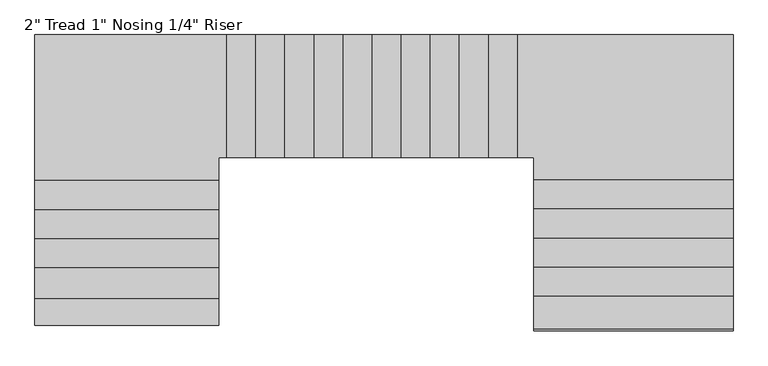
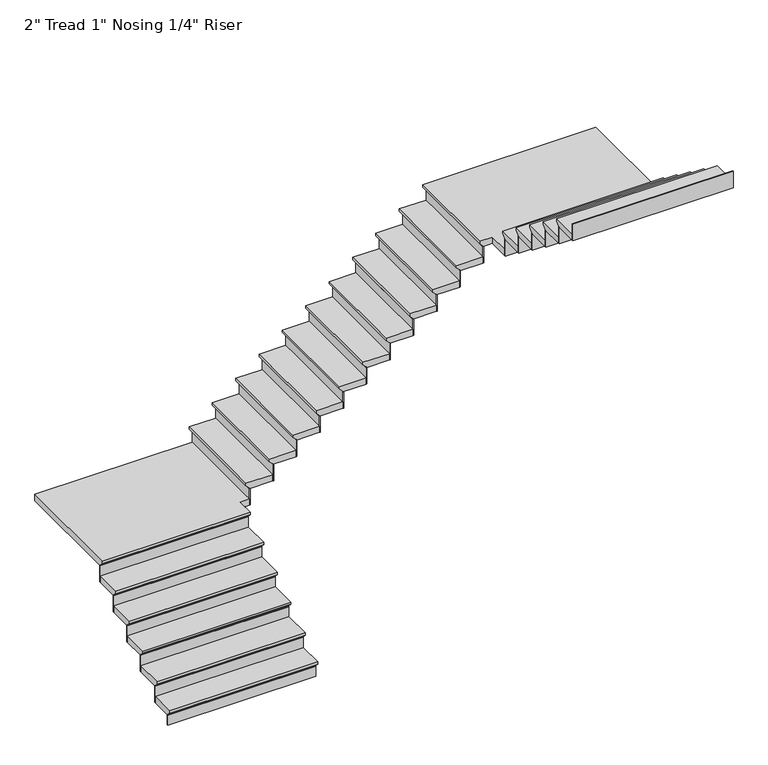
"""IFC4 building model written with IfcOpenShell, lengths in millimetres: stair flight geometry."""

from ifc_helpers import new_model, si_unit, origin, place, context, project, spatial, faceted_brep, source, transform, mapped, element, save


def stair_flight_d1d5caa0(model_context):
    return source(origin(), model_context, "Body", "Brep", [
        faceted_brep([(-2368.6972892, 4718.9167606, 3313.8717391), (-2368.6972892, 4718.9167606, 3332.9217391), (-3493.0046642, 4718.9167606, 3332.9217391), (-3493.0046642, 4718.9167606, 3313.8717391), (-2368.6972892, 4744.3167606, 3288.4717391), (-3493.0046642, 4744.3167606, 3288.4717391), (-2368.6972892, 4909.4167606, 3332.9217391), (-3493.0046642, 4909.4167606, 3332.9217391), (-3493.0046642, 4744.3167606, 3282.1217391), (-3493.0046642, 4909.4167606, 3282.1217391), (-2368.6972892, 4909.4167606, 3282.1217391), (-2368.6972892, 4744.3167606, 3282.1217391)], [[[0, 1, 2, 3]], [[4, 0, 3, 5]], [[2, 1, 6, 7]], [[8, 9, 10, 11]], [[2, 7, 9, 8, 5, 3]], [[8, 11, 4, 5]], [[6, 1, 0, 4, 11, 10]], [[7, 6, 10, 9]]]),
        faceted_brep([(-2368.6972892, 4744.3167606, 3282.1217391), (-2368.6972892, 4744.3167606, 3200.4), (-2368.6972892, 4750.6667606, 3200.4), (-2368.6972892, 4750.6667606, 3282.1217391), (-3493.0046642, 4744.3167606, 3282.1217391), (-3493.0046642, 4750.6667606, 3282.1217391), (-3493.0046642, 4750.6667606, 3200.4), (-3493.0046642, 4744.3167606, 3200.4)], [[[0, 1, 2, 3]], [[4, 5, 6, 7]], [[1, 0, 4, 7]], [[2, 1, 7, 6]], [[3, 2, 6, 5]], [[0, 3, 5, 4]]]),
        faceted_brep([(-2368.6972892, 4909.4167606, 3414.6434783), (-2368.6972892, 4909.4167606, 3282.1217391), (-2368.6972892, 4915.7667606, 3282.1217391), (-2368.6972892, 4915.7667606, 3414.6434783), (-3493.0046642, 4909.4167606, 3414.6434783), (-3493.0046642, 4915.7667606, 3414.6434783), (-3493.0046642, 4915.7667606, 3282.1217391), (-3493.0046642, 4909.4167606, 3282.1217391)], [[[0, 1, 2, 3]], [[4, 5, 6, 7]], [[1, 0, 4, 7]], [[2, 1, 7, 6]], [[3, 2, 6, 5]], [[0, 3, 5, 4]]]),
        faceted_brep([(-3493.0046642, 4884.0167606, 3465.4434783), (-2368.6972892, 4884.0167606, 3465.4434783), (-2368.6972892, 5099.9164494, 3465.4434783), (-3493.0046642, 5099.9164494, 3465.4434783), (-3493.0046642, 4909.4167606, 3414.6434783), (-3493.0046642, 5099.9164494, 3414.6434783), (-2368.6972892, 5099.9164494, 3414.6434783), (-2368.6972892, 4909.4167606, 3414.6434783), (-3493.0046642, 4909.4167606, 3420.9934783), (-3493.0046642, 4884.0167606, 3446.3934783), (-2368.6972892, 4909.4167606, 3420.9934783), (-2368.6972892, 4884.0167606, 3446.3934783)], [[[0, 1, 2, 3]], [[4, 5, 6, 7]], [[0, 3, 5, 4, 8, 9]], [[4, 7, 10, 8]], [[2, 1, 11, 10, 7, 6]], [[3, 2, 6, 5]], [[11, 1, 0, 9]], [[10, 11, 9, 8]]]),
        faceted_brep([(-2368.6972892, 5099.9164494, 3547.1652174), (-2368.6972892, 5099.9164494, 3414.6434783), (-2368.6972892, 5106.2664494, 3414.6434783), (-2368.6972892, 5106.2664494, 3547.1652174), (-3493.0046642, 5099.9164494, 3547.1652174), (-3493.0046642, 5106.2664494, 3547.1652174), (-3493.0046642, 5106.2664494, 3414.6434783), (-3493.0046642, 5099.9164494, 3414.6434783)], [[[0, 1, 2, 3]], [[4, 5, 6, 7]], [[1, 0, 4, 7]], [[2, 1, 7, 6]], [[3, 2, 6, 5]], [[0, 3, 5, 4]]]),
        faceted_brep([(-3493.0046642, 5074.5164494, 3597.9652174), (-2368.6972892, 5074.5164494, 3597.9652174), (-2368.6972892, 5277.7164494, 3597.9652174), (-3493.0046642, 5277.7164494, 3597.9652174), (-3493.0046642, 5099.9164494, 3547.1652174), (-3493.0046642, 5277.7164494, 3547.1652174), (-2368.6972892, 5277.7164494, 3547.1652174), (-2368.6972892, 5099.9164494, 3547.1652174), (-3493.0046642, 5099.9164494, 3553.5152174), (-3493.0046642, 5074.5164494, 3578.9152174), (-2368.6972892, 5099.9164494, 3553.5152174), (-2368.6972892, 5074.5164494, 3578.9152174)], [[[0, 1, 2, 3]], [[4, 5, 6, 7]], [[0, 3, 5, 4, 8, 9]], [[4, 7, 10, 8]], [[2, 1, 11, 10, 7, 6]], [[3, 2, 6, 5]], [[11, 1, 0, 9]], [[10, 11, 9, 8]]]),
        faceted_brep([(-2368.6972892, 5277.7164494, 3679.6869565), (-2368.6972892, 5277.7164494, 3547.1652174), (-2368.6972892, 5284.0664494, 3547.1652174), (-2368.6972892, 5284.0664494, 3679.6869565), (-3493.0046642, 5277.7164494, 3679.6869565), (-3493.0046642, 5284.0664494, 3679.6869565), (-3493.0046642, 5284.0664494, 3547.1652174), (-3493.0046642, 5277.7164494, 3547.1652174)], [[[0, 1, 2, 3]], [[4, 5, 6, 7]], [[1, 0, 4, 7]], [[2, 1, 7, 6]], [[3, 2, 6, 5]], [[0, 3, 5, 4]]]),
        faceted_brep([(-3493.0046642, 5252.3164494, 3730.4869565), (-2368.6972892, 5252.3164494, 3730.4869565), (-2368.6972892, 5455.5164494, 3730.4869565), (-3493.0046642, 5455.5164494, 3730.4869565), (-3493.0046642, 5277.7164494, 3679.6869565), (-3493.0046642, 5455.5164494, 3679.6869565), (-2368.6972892, 5455.5164494, 3679.6869565), (-2368.6972892, 5277.7164494, 3679.6869565), (-3493.0046642, 5277.7164494, 3686.0369565), (-3493.0046642, 5252.3164494, 3711.4369565), (-2368.6972892, 5277.7164494, 3686.0369565), (-2368.6972892, 5252.3164494, 3711.4369565)], [[[0, 1, 2, 3]], [[4, 5, 6, 7]], [[0, 3, 5, 4, 8, 9]], [[4, 7, 10, 8]], [[2, 1, 11, 10, 7, 6]], [[3, 2, 6, 5]], [[11, 1, 0, 9]], [[10, 11, 9, 8]]]),
        faceted_brep([(-2368.6972892, 5455.5164494, 3812.2086957), (-2368.6972892, 5455.5164494, 3679.6869565), (-2368.6972892, 5461.8664494, 3679.6869565), (-2368.6972892, 5461.8664494, 3812.2086957), (-3493.0046642, 5455.5164494, 3812.2086957), (-3493.0046642, 5461.8664494, 3812.2086957), (-3493.0046642, 5461.8664494, 3679.6869565), (-3493.0046642, 5455.5164494, 3679.6869565)], [[[0, 1, 2, 3]], [[4, 5, 6, 7]], [[1, 0, 4, 7]], [[2, 1, 7, 6]], [[3, 2, 6, 5]], [[0, 3, 5, 4]]]),
        faceted_brep([(-3493.0046642, 5430.1164494, 3863.0086957), (-2368.6972892, 5430.1164494, 3863.0086957), (-2368.6972892, 5633.3167606, 3863.0086957), (-3493.0046642, 5633.3167606, 3863.0086957), (-3493.0046642, 5455.5164494, 3812.2086957), (-3493.0046642, 5633.3167606, 3812.2086957), (-2368.6972892, 5633.3167606, 3812.2086957), (-2368.6972892, 5455.5164494, 3812.2086957), (-3493.0046642, 5455.5164494, 3818.5586957), (-3493.0046642, 5430.1164494, 3843.9586957), (-2368.6972892, 5455.5164494, 3818.5586957), (-2368.6972892, 5430.1164494, 3843.9586957)], [[[0, 1, 2, 3]], [[4, 5, 6, 7]], [[0, 3, 5, 4, 8, 9]], [[4, 7, 10, 8]], [[2, 1, 11, 10, 7, 6]], [[3, 2, 6, 5]], [[11, 1, 0, 9]], [[10, 11, 9, 8]]]),
        faceted_brep([(-2368.6972892, 5633.3167606, 3944.7304348), (-2368.6972892, 5633.3167606, 3812.2086957), (-2368.6972892, 5639.6667606, 3812.2086957), (-2368.6972892, 5639.6667606, 3944.7304348), (-3493.0046642, 5633.3167606, 3944.7304348), (-3493.0046642, 5639.6667606, 3944.7304348), (-3493.0046642, 5639.6667606, 3812.2086957), (-3493.0046642, 5633.3167606, 3812.2086957)], [[[0, 1, 2, 3]], [[4, 5, 6, 7]], [[1, 0, 4, 7]], [[2, 1, 7, 6]], [[3, 2, 6, 5]], [[0, 3, 5, 4]]]),
        faceted_brep([(-2295.032382, 6496.9167606, 3995.5304348), (-3493.0046642, 6496.9167606, 3995.5304348), (-3493.0046642, 5607.9167606, 3995.5304348), (-2368.6972892, 5607.9167606, 3995.5304348), (-2368.6972892, 5746.5536537, 3995.5304348), (-2295.032382, 5746.5536537, 3995.5304348), (-3493.0046642, 6496.9167606, 3944.7304348), (-2295.032382, 6496.9167606, 3944.7304348), (-2295.032382, 5746.5536537, 3944.7304348), (-2368.6972892, 5746.5536537, 3944.7304348), (-2368.6972892, 5633.3167606, 3944.7304348), (-3493.0046642, 5633.3167606, 3944.7304348), (-3493.0046642, 5633.3167606, 3951.0804348), (-3493.0046642, 5607.9167606, 3976.4804348), (-2368.6972892, 5633.3167606, 3951.0804348), (-2368.6972892, 5607.9167606, 3976.4804348)], [[[0, 1, 2, 3, 4, 5]], [[6, 7, 8, 9, 10, 11]], [[1, 0, 7, 6]], [[2, 1, 6, 11, 12, 13]], [[11, 10, 14, 12]], [[4, 3, 15, 14, 10, 9]], [[5, 4, 9, 8]], [[0, 5, 8, 7]], [[15, 3, 2, 13]], [[14, 15, 13, 12]]]),
        faceted_brep([(-2295.032382, 5746.5536537, 4077.2521739), (-2295.032382, 5746.5536537, 3944.7304348), (-2288.682382, 5746.5536537, 3944.7304348), (-2288.682382, 5746.5536537, 4077.2521739), (-2295.032382, 6496.9167606, 4077.2521739), (-2288.682382, 6496.9167606, 4077.2521739), (-2288.682382, 6496.9167606, 3944.7304348), (-2295.032382, 6496.9167606, 3944.7304348)], [[[0, 1, 2, 3]], [[4, 5, 6, 7]], [[1, 0, 4, 7]], [[2, 1, 7, 6]], [[3, 2, 6, 5]], [[0, 3, 5, 4]]]),
        faceted_brep([(-2320.432382, 6496.9167606, 4128.0521739), (-2320.432382, 5746.5536537, 4128.0521739), (-2117.232382, 5746.5536537, 4128.0521739), (-2117.232382, 6496.9167606, 4128.0521739), (-2295.032382, 6496.9167606, 4077.2521739), (-2117.232382, 6496.9167606, 4077.2521739), (-2117.232382, 5746.5536537, 4077.2521739), (-2295.032382, 5746.5536537, 4077.2521739), (-2295.032382, 6496.9167606, 4083.6021739), (-2320.432382, 6496.9167606, 4109.0021739), (-2295.032382, 5746.5536537, 4083.6021739), (-2320.432382, 5746.5536537, 4109.0021739)], [[[0, 1, 2, 3]], [[4, 5, 6, 7]], [[0, 3, 5, 4, 8, 9]], [[4, 7, 10, 8]], [[2, 1, 11, 10, 7, 6]], [[3, 2, 6, 5]], [[11, 1, 0, 9]], [[10, 11, 9, 8]]]),
        faceted_brep([(-2117.232382, 5746.5536537, 4209.773913), (-2117.232382, 5746.5536537, 4077.2521739), (-2110.882382, 5746.5536537, 4077.2521739), (-2110.882382, 5746.5536537, 4209.773913), (-2117.232382, 6496.9167606, 4209.773913), (-2110.882382, 6496.9167606, 4209.773913), (-2110.882382, 6496.9167606, 4077.2521739), (-2117.232382, 6496.9167606, 4077.2521739)], [[[0, 1, 2, 3]], [[4, 5, 6, 7]], [[1, 0, 4, 7]], [[2, 1, 7, 6]], [[3, 2, 6, 5]], [[0, 3, 5, 4]]]),
        faceted_brep([(-2142.632382, 6496.9167606, 4260.573913), (-2142.632382, 5746.5536537, 4260.573913), (-1939.432382, 5746.5536537, 4260.573913), (-1939.432382, 6496.9167606, 4260.573913), (-2117.232382, 6496.9167606, 4209.773913), (-1939.432382, 6496.9167606, 4209.773913), (-1939.432382, 5746.5536537, 4209.773913), (-2117.232382, 5746.5536537, 4209.773913), (-2117.232382, 6496.9167606, 4216.123913), (-2142.632382, 6496.9167606, 4241.523913), (-2117.232382, 5746.5536537, 4216.123913), (-2142.632382, 5746.5536537, 4241.523913)], [[[0, 1, 2, 3]], [[4, 5, 6, 7]], [[0, 3, 5, 4, 8, 9]], [[4, 7, 10, 8]], [[2, 1, 11, 10, 7, 6]], [[3, 2, 6, 5]], [[11, 1, 0, 9]], [[10, 11, 9, 8]]]),
        faceted_brep([(-1939.432382, 5746.5536537, 4342.2956522), (-1939.432382, 5746.5536537, 4209.773913), (-1933.082382, 5746.5536537, 4209.773913), (-1933.082382, 5746.5536537, 4342.2956522), (-1939.432382, 6496.9167606, 4342.2956522), (-1933.082382, 6496.9167606, 4342.2956522), (-1933.082382, 6496.9167606, 4209.773913), (-1939.432382, 6496.9167606, 4209.773913)], [[[0, 1, 2, 3]], [[4, 5, 6, 7]], [[1, 0, 4, 7]], [[2, 1, 7, 6]], [[3, 2, 6, 5]], [[0, 3, 5, 4]]]),
        faceted_brep([(-1964.832382, 6496.9167606, 4393.0956522), (-1964.832382, 5746.5536537, 4393.0956522), (-1761.632382, 5746.5536537, 4393.0956522), (-1761.632382, 6496.9167606, 4393.0956522), (-1939.432382, 6496.9167606, 4342.2956522), (-1761.632382, 6496.9167606, 4342.2956522), (-1761.632382, 5746.5536537, 4342.2956522), (-1939.432382, 5746.5536537, 4342.2956522), (-1939.432382, 6496.9167606, 4348.6456522), (-1964.832382, 6496.9167606, 4374.0456522), (-1939.432382, 5746.5536537, 4348.6456522), (-1964.832382, 5746.5536537, 4374.0456522)], [[[0, 1, 2, 3]], [[4, 5, 6, 7]], [[0, 3, 5, 4, 8, 9]], [[4, 7, 10, 8]], [[2, 1, 11, 10, 7, 6]], [[3, 2, 6, 5]], [[11, 1, 0, 9]], [[10, 11, 9, 8]]]),
        faceted_brep([(-1761.632382, 5746.5536537, 4474.8173913), (-1761.632382, 5746.5536537, 4342.2956522), (-1755.282382, 5746.5536537, 4342.2956522), (-1755.282382, 5746.5536537, 4474.8173913), (-1761.632382, 6496.9167606, 4474.8173913), (-1755.282382, 6496.9167606, 4474.8173913), (-1755.282382, 6496.9167606, 4342.2956522), (-1761.632382, 6496.9167606, 4342.2956522)], [[[0, 1, 2, 3]], [[4, 5, 6, 7]], [[1, 0, 4, 7]], [[2, 1, 7, 6]], [[3, 2, 6, 5]], [[0, 3, 5, 4]]]),
        faceted_brep([(-1787.032382, 6496.9167606, 4525.6173913), (-1787.032382, 5746.5536537, 4525.6173913), (-1583.832382, 5746.5536537, 4525.6173913), (-1583.832382, 6496.9167606, 4525.6173913), (-1761.632382, 6496.9167606, 4474.8173913), (-1583.832382, 6496.9167606, 4474.8173913), (-1583.832382, 5746.5536537, 4474.8173913), (-1761.632382, 5746.5536537, 4474.8173913), (-1761.632382, 6496.9167606, 4481.1673913), (-1787.032382, 6496.9167606, 4506.5673913), (-1761.632382, 5746.5536537, 4481.1673913), (-1787.032382, 5746.5536537, 4506.5673913)], [[[0, 1, 2, 3]], [[4, 5, 6, 7]], [[0, 3, 5, 4, 8, 9]], [[4, 7, 10, 8]], [[2, 1, 11, 10, 7, 6]], [[3, 2, 6, 5]], [[11, 1, 0, 9]], [[10, 11, 9, 8]]]),
        faceted_brep([(-1583.832382, 5746.5536537, 4607.3391304), (-1583.832382, 5746.5536537, 4474.8173913), (-1577.482382, 5746.5536537, 4474.8173913), (-1577.482382, 5746.5536537, 4607.3391304), (-1583.832382, 6496.9167606, 4607.3391304), (-1577.482382, 6496.9167606, 4607.3391304), (-1577.482382, 6496.9167606, 4474.8173913), (-1583.832382, 6496.9167606, 4474.8173913)], [[[0, 1, 2, 3]], [[4, 5, 6, 7]], [[1, 0, 4, 7]], [[2, 1, 7, 6]], [[3, 2, 6, 5]], [[0, 3, 5, 4]]]),
        faceted_brep([(-1609.232382, 6496.9167606, 4658.1391304), (-1609.232382, 5746.5536537, 4658.1391304), (-1406.032382, 5746.5536537, 4658.1391304), (-1406.032382, 6496.9167606, 4658.1391304), (-1583.832382, 6496.9167606, 4607.3391304), (-1406.032382, 6496.9167606, 4607.3391304), (-1406.032382, 5746.5536537, 4607.3391304), (-1583.832382, 5746.5536537, 4607.3391304), (-1583.832382, 6496.9167606, 4613.6891304), (-1609.232382, 6496.9167606, 4639.0891304), (-1583.832382, 5746.5536537, 4613.6891304), (-1609.232382, 5746.5536537, 4639.0891304)], [[[0, 1, 2, 3]], [[4, 5, 6, 7]], [[0, 3, 5, 4, 8, 9]], [[4, 7, 10, 8]], [[2, 1, 11, 10, 7, 6]], [[3, 2, 6, 5]], [[11, 1, 0, 9]], [[10, 11, 9, 8]]]),
        faceted_brep([(-1406.032382, 5746.5536537, 4739.8608696), (-1406.032382, 5746.5536537, 4607.3391304), (-1399.682382, 5746.5536537, 4607.3391304), (-1399.682382, 5746.5536537, 4739.8608696), (-1406.032382, 6496.9167606, 4739.8608696), (-1399.682382, 6496.9167606, 4739.8608696), (-1399.682382, 6496.9167606, 4607.3391304), (-1406.032382, 6496.9167606, 4607.3391304)], [[[0, 1, 2, 3]], [[4, 5, 6, 7]], [[1, 0, 4, 7]], [[2, 1, 7, 6]], [[3, 2, 6, 5]], [[0, 3, 5, 4]]]),
        faceted_brep([(-1431.432382, 6496.9167606, 4790.6608696), (-1431.432382, 5746.5536537, 4790.6608696), (-1228.232382, 5746.5536537, 4790.6608696), (-1228.232382, 6496.9167606, 4790.6608696), (-1406.032382, 6496.9167606, 4739.8608696), (-1228.232382, 6496.9167606, 4739.8608696), (-1228.232382, 5746.5536537, 4739.8608696), (-1406.032382, 5746.5536537, 4739.8608696), (-1406.032382, 6496.9167606, 4746.2108696), (-1431.432382, 6496.9167606, 4771.6108696), (-1406.032382, 5746.5536537, 4746.2108696), (-1431.432382, 5746.5536537, 4771.6108696)], [[[0, 1, 2, 3]], [[4, 5, 6, 7]], [[0, 3, 5, 4, 8, 9]], [[4, 7, 10, 8]], [[2, 1, 11, 10, 7, 6]], [[3, 2, 6, 5]], [[11, 1, 0, 9]], [[10, 11, 9, 8]]]),
        faceted_brep([(-1228.232382, 5746.5536537, 4872.3826087), (-1228.232382, 5746.5536537, 4739.8608696), (-1221.882382, 5746.5536537, 4739.8608696), (-1221.882382, 5746.5536537, 4872.3826087), (-1228.232382, 6496.9167606, 4872.3826087), (-1221.882382, 6496.9167606, 4872.3826087), (-1221.882382, 6496.9167606, 4739.8608696), (-1228.232382, 6496.9167606, 4739.8608696)], [[[0, 1, 2, 3]], [[4, 5, 6, 7]], [[1, 0, 4, 7]], [[2, 1, 7, 6]], [[3, 2, 6, 5]], [[0, 3, 5, 4]]]),
        faceted_brep([(-1253.632382, 6496.9167606, 4923.1826087), (-1253.632382, 5746.5536537, 4923.1826087), (-1050.432382, 5746.5536537, 4923.1826087), (-1050.432382, 6496.9167606, 4923.1826087), (-1228.232382, 6496.9167606, 4872.3826087), (-1050.432382, 6496.9167606, 4872.3826087), (-1050.432382, 5746.5536537, 4872.3826087), (-1228.232382, 5746.5536537, 4872.3826087), (-1228.232382, 6496.9167606, 4878.7326087), (-1253.632382, 6496.9167606, 4904.1326087), (-1228.232382, 5746.5536537, 4878.7326087), (-1253.632382, 5746.5536537, 4904.1326087)], [[[0, 1, 2, 3]], [[4, 5, 6, 7]], [[0, 3, 5, 4, 8, 9]], [[4, 7, 10, 8]], [[2, 1, 11, 10, 7, 6]], [[3, 2, 6, 5]], [[11, 1, 0, 9]], [[10, 11, 9, 8]]]),
        faceted_brep([(-1050.432382, 5746.5536537, 5004.9043478), (-1050.432382, 5746.5536537, 4872.3826087), (-1044.082382, 5746.5536537, 4872.3826087), (-1044.082382, 5746.5536537, 5004.9043478), (-1050.432382, 6496.9167606, 5004.9043478), (-1044.082382, 6496.9167606, 5004.9043478), (-1044.082382, 6496.9167606, 4872.3826087), (-1050.432382, 6496.9167606, 4872.3826087)], [[[0, 1, 2, 3]], [[4, 5, 6, 7]], [[1, 0, 4, 7]], [[2, 1, 7, 6]], [[3, 2, 6, 5]], [[0, 3, 5, 4]]]),
        faceted_brep([(-1075.832382, 6496.9167606, 5055.7043478), (-1075.832382, 5746.5536537, 5055.7043478), (-872.632382, 5746.5536537, 5055.7043478), (-872.632382, 6496.9167606, 5055.7043478), (-1050.432382, 6496.9167606, 5004.9043478), (-872.632382, 6496.9167606, 5004.9043478), (-872.632382, 5746.5536537, 5004.9043478), (-1050.432382, 5746.5536537, 5004.9043478), (-1050.432382, 6496.9167606, 5011.2543478), (-1075.832382, 6496.9167606, 5036.6543478), (-1050.432382, 5746.5536537, 5011.2543478), (-1075.832382, 5746.5536537, 5036.6543478)], [[[0, 1, 2, 3]], [[4, 5, 6, 7]], [[0, 3, 5, 4, 8, 9]], [[4, 7, 10, 8]], [[2, 1, 11, 10, 7, 6]], [[3, 2, 6, 5]], [[11, 1, 0, 9]], [[10, 11, 9, 8]]]),
        faceted_brep([(-872.632382, 5746.5536537, 5137.426087), (-872.632382, 5746.5536537, 5004.9043478), (-866.282382, 5746.5536537, 5004.9043478), (-866.282382, 5746.5536537, 5137.426087), (-872.632382, 6496.9167606, 5137.426087), (-866.282382, 6496.9167606, 5137.426087), (-866.282382, 6496.9167606, 5004.9043478), (-872.632382, 6496.9167606, 5004.9043478)], [[[0, 1, 2, 3]], [[4, 5, 6, 7]], [[1, 0, 4, 7]], [[2, 1, 7, 6]], [[3, 2, 6, 5]], [[0, 3, 5, 4]]]),
        faceted_brep([(-898.032382, 6496.9167606, 5188.226087), (-898.032382, 5746.5536537, 5188.226087), (-694.832382, 5746.5536537, 5188.226087), (-694.832382, 6496.9167606, 5188.226087), (-872.632382, 6496.9167606, 5137.426087), (-694.832382, 6496.9167606, 5137.426087), (-694.832382, 5746.5536537, 5137.426087), (-872.632382, 5746.5536537, 5137.426087), (-872.632382, 6496.9167606, 5143.776087), (-898.032382, 6496.9167606, 5169.176087), (-872.632382, 5746.5536537, 5143.776087), (-898.032382, 5746.5536537, 5169.176087)], [[[0, 1, 2, 3]], [[4, 5, 6, 7]], [[0, 3, 5, 4, 8, 9]], [[4, 7, 10, 8]], [[2, 1, 11, 10, 7, 6]], [[3, 2, 6, 5]], [[11, 1, 0, 9]], [[10, 11, 9, 8]]]),
        faceted_brep([(-694.832382, 5746.5536537, 5269.9478261), (-694.832382, 5746.5536537, 5137.426087), (-688.482382, 5746.5536537, 5137.426087), (-688.482382, 5746.5536537, 5269.9478261), (-694.832382, 6496.9167606, 5269.9478261), (-688.482382, 6496.9167606, 5269.9478261), (-688.482382, 6496.9167606, 5137.426087), (-694.832382, 6496.9167606, 5137.426087)], [[[0, 1, 2, 3]], [[4, 5, 6, 7]], [[1, 0, 4, 7]], [[2, 1, 7, 6]], [[3, 2, 6, 5]], [[0, 3, 5, 4]]]),
        faceted_brep([(-720.232382, 6496.9167606, 5320.7478261), (-720.232382, 5746.5536537, 5320.7478261), (-517.032382, 5746.5536537, 5320.7478261), (-517.032382, 6496.9167606, 5320.7478261), (-694.832382, 6496.9167606, 5269.9478261), (-517.032382, 6496.9167606, 5269.9478261), (-517.032382, 5746.5536537, 5269.9478261), (-694.832382, 5746.5536537, 5269.9478261), (-694.832382, 6496.9167606, 5276.2978261), (-720.232382, 6496.9167606, 5301.6978261), (-694.832382, 5746.5536537, 5276.2978261), (-720.232382, 5746.5536537, 5301.6978261)], [[[0, 1, 2, 3]], [[4, 5, 6, 7]], [[0, 3, 5, 4, 8, 9]], [[4, 7, 10, 8]], [[2, 1, 11, 10, 7, 6]], [[3, 2, 6, 5]], [[11, 1, 0, 9]], [[10, 11, 9, 8]]]),
        faceted_brep([(-517.032382, 5746.5536537, 5402.4695652), (-517.032382, 5746.5536537, 5269.9478261), (-510.682382, 5746.5536537, 5269.9478261), (-510.682382, 5746.5536537, 5402.4695652), (-517.032382, 6496.9167606, 5402.4695652), (-510.682382, 6496.9167606, 5402.4695652), (-510.682382, 6496.9167606, 5269.9478261), (-517.032382, 6496.9167606, 5269.9478261)], [[[0, 1, 2, 3]], [[4, 5, 6, 7]], [[1, 0, 4, 7]], [[2, 1, 7, 6]], [[3, 2, 6, 5]], [[0, 3, 5, 4]]]),
        faceted_brep([(774.1953358, 5582.5167606, 5453.2695652), (774.1953358, 6496.9167606, 5453.2695652), (-542.432382, 6496.9167606, 5453.2695652), (-542.432382, 5746.5536537, 5453.2695652), (-445.0046642, 5746.5536537, 5453.2695652), (-445.0046642, 5582.5167606, 5453.2695652), (774.1953358, 6496.9167606, 5402.4695652), (774.1953358, 5582.5167606, 5402.4695652), (-445.0046642, 5582.5167606, 5402.4695652), (-445.0046642, 5746.5536537, 5402.4695652), (-517.032382, 5746.5536537, 5402.4695652), (-517.032382, 6496.9167606, 5402.4695652), (-517.032382, 6496.9167606, 5408.8195652), (-542.432382, 6496.9167606, 5434.2195652), (-517.032382, 5746.5536537, 5408.8195652), (-542.432382, 5746.5536537, 5434.2195652)], [[[0, 1, 2, 3, 4, 5]], [[6, 7, 8, 9, 10, 11]], [[1, 0, 7, 6]], [[2, 1, 6, 11, 12, 13]], [[11, 10, 14, 12]], [[4, 3, 15, 14, 10, 9]], [[5, 4, 9, 8]], [[0, 5, 8, 7]], [[15, 3, 2, 13]], [[14, 15, 13, 12]]]),
        faceted_brep([(-445.0046642, 5582.5167606, 5534.9913043), (-445.0046642, 5582.5167606, 5402.4695652), (-445.0046642, 5576.1667606, 5402.4695652), (-445.0046642, 5576.1667606, 5534.9913043), (774.1953358, 5582.5167606, 5534.9913043), (774.1953358, 5576.1667606, 5534.9913043), (774.1953358, 5576.1667606, 5402.4695652), (774.1953358, 5582.5167606, 5402.4695652)], [[[0, 1, 2, 3]], [[4, 5, 6, 7]], [[1, 0, 4, 7]], [[2, 1, 7, 6]], [[3, 2, 6, 5]], [[0, 3, 5, 4]]]),
        faceted_brep([(774.1953358, 5607.9167606, 5585.7913043), (-445.0046642, 5607.9167606, 5585.7913043), (-445.0046642, 5404.7164494, 5585.7913043), (774.1953358, 5404.7164494, 5585.7913043), (774.1953358, 5582.5167606, 5534.9913043), (774.1953358, 5404.7164494, 5534.9913043), (-445.0046642, 5404.7164494, 5534.9913043), (-445.0046642, 5582.5167606, 5534.9913043), (774.1953358, 5582.5167606, 5541.3413043), (774.1953358, 5607.9167606, 5566.7413043), (-445.0046642, 5582.5167606, 5541.3413043), (-445.0046642, 5607.9167606, 5566.7413043)], [[[0, 1, 2, 3]], [[4, 5, 6, 7]], [[0, 3, 5, 4, 8, 9]], [[4, 7, 10, 8]], [[2, 1, 11, 10, 7, 6]], [[3, 2, 6, 5]], [[11, 1, 0, 9]], [[10, 11, 9, 8]]]),
        faceted_brep([(-445.0046642, 5404.7164494, 5667.5130435), (-445.0046642, 5404.7164494, 5534.9913043), (-445.0046642, 5398.3664494, 5534.9913043), (-445.0046642, 5398.3664494, 5667.5130435), (774.1953358, 5404.7164494, 5667.5130435), (774.1953358, 5398.3664494, 5667.5130435), (774.1953358, 5398.3664494, 5534.9913043), (774.1953358, 5404.7164494, 5534.9913043)], [[[0, 1, 2, 3]], [[4, 5, 6, 7]], [[1, 0, 4, 7]], [[2, 1, 7, 6]], [[3, 2, 6, 5]], [[0, 3, 5, 4]]]),
        faceted_brep([(774.1953358, 5430.1164494, 5718.3130435), (-445.0046642, 5430.1164494, 5718.3130435), (-445.0046642, 5226.9164494, 5718.3130435), (774.1953358, 5226.9164494, 5718.3130435), (774.1953358, 5404.7164494, 5667.5130435), (774.1953358, 5226.9164494, 5667.5130435), (-445.0046642, 5226.9164494, 5667.5130435), (-445.0046642, 5404.7164494, 5667.5130435), (774.1953358, 5404.7164494, 5673.8630435), (774.1953358, 5430.1164494, 5699.2630435), (-445.0046642, 5404.7164494, 5673.8630435), (-445.0046642, 5430.1164494, 5699.2630435)], [[[0, 1, 2, 3]], [[4, 5, 6, 7]], [[0, 3, 5, 4, 8, 9]], [[4, 7, 10, 8]], [[2, 1, 11, 10, 7, 6]], [[3, 2, 6, 5]], [[11, 1, 0, 9]], [[10, 11, 9, 8]]]),
        faceted_brep([(-445.0046642, 5226.9164494, 5800.0347826), (-445.0046642, 5226.9164494, 5667.5130435), (-445.0046642, 5220.5664494, 5667.5130435), (-445.0046642, 5220.5664494, 5800.0347826), (774.1953358, 5226.9164494, 5800.0347826), (774.1953358, 5220.5664494, 5800.0347826), (774.1953358, 5220.5664494, 5667.5130435), (774.1953358, 5226.9164494, 5667.5130435)], [[[0, 1, 2, 3]], [[4, 5, 6, 7]], [[1, 0, 4, 7]], [[2, 1, 7, 6]], [[3, 2, 6, 5]], [[0, 3, 5, 4]]]),
        faceted_brep([(774.1953358, 5252.3164494, 5850.8347826), (-445.0046642, 5252.3164494, 5850.8347826), (-445.0046642, 5049.1164494, 5850.8347826), (774.1953358, 5049.1164494, 5850.8347826), (774.1953358, 5226.9164494, 5800.0347826), (774.1953358, 5049.1164494, 5800.0347826), (-445.0046642, 5049.1164494, 5800.0347826), (-445.0046642, 5226.9164494, 5800.0347826), (774.1953358, 5226.9164494, 5806.3847826), (774.1953358, 5252.3164494, 5831.7847826), (-445.0046642, 5226.9164494, 5806.3847826), (-445.0046642, 5252.3164494, 5831.7847826)], [[[0, 1, 2, 3]], [[4, 5, 6, 7]], [[0, 3, 5, 4, 8, 9]], [[4, 7, 10, 8]], [[2, 1, 11, 10, 7, 6]], [[3, 2, 6, 5]], [[11, 1, 0, 9]], [[10, 11, 9, 8]]]),
        faceted_brep([(-445.0046642, 5049.1164494, 5932.5565217), (-445.0046642, 5049.1164494, 5800.0347826), (-445.0046642, 5042.7664494, 5800.0347826), (-445.0046642, 5042.7664494, 5932.5565217), (774.1953358, 5049.1164494, 5932.5565217), (774.1953358, 5042.7664494, 5932.5565217), (774.1953358, 5042.7664494, 5800.0347826), (774.1953358, 5049.1164494, 5800.0347826)], [[[0, 1, 2, 3]], [[4, 5, 6, 7]], [[1, 0, 4, 7]], [[2, 1, 7, 6]], [[3, 2, 6, 5]], [[0, 3, 5, 4]]]),
        faceted_brep([(774.1953358, 5074.5164494, 5983.3565217), (-445.0046642, 5074.5164494, 5983.3565217), (-445.0046642, 4871.3164494, 5983.3565217), (774.1953358, 4871.3164494, 5983.3565217), (774.1953358, 5049.1164494, 5932.5565217), (774.1953358, 4871.3164494, 5932.5565217), (-445.0046642, 4871.3164494, 5932.5565217), (-445.0046642, 5049.1164494, 5932.5565217), (774.1953358, 5049.1164494, 5938.9065217), (774.1953358, 5074.5164494, 5964.3065217), (-445.0046642, 5049.1164494, 5938.9065217), (-445.0046642, 5074.5164494, 5964.3065217)], [[[0, 1, 2, 3]], [[4, 5, 6, 7]], [[0, 3, 5, 4, 8, 9]], [[4, 7, 10, 8]], [[2, 1, 11, 10, 7, 6]], [[3, 2, 6, 5]], [[11, 1, 0, 9]], [[10, 11, 9, 8]]]),
        faceted_brep([(-445.0046642, 4871.3164494, 6065.0782609), (-445.0046642, 4871.3164494, 5932.5565217), (-445.0046642, 4864.9664494, 5932.5565217), (-445.0046642, 4864.9664494, 6065.0782609), (774.1953358, 4871.3164494, 6065.0782609), (774.1953358, 4864.9664494, 6065.0782609), (774.1953358, 4864.9664494, 5932.5565217), (774.1953358, 4871.3164494, 5932.5565217)], [[[0, 1, 2, 3]], [[4, 5, 6, 7]], [[1, 0, 4, 7]], [[2, 1, 7, 6]], [[3, 2, 6, 5]], [[0, 3, 5, 4]]]),
        faceted_brep([(-445.0046642, 4693.5167606, 6197.6), (-445.0046642, 4693.5167606, 6065.0782609), (-445.0046642, 4687.1667606, 6065.0782609), (-445.0046642, 4687.1667606, 6197.6), (774.1953358, 4693.5167606, 6197.6), (774.1953358, 4687.1667606, 6197.6), (774.1953358, 4687.1667606, 6065.0782609), (774.1953358, 4693.5167606, 6065.0782609)], [[[0, 1, 2, 3]], [[4, 5, 6, 7]], [[1, 0, 4, 7]], [[2, 1, 7, 6]], [[3, 2, 6, 5]], [[0, 3, 5, 4]]]),
        faceted_brep([(774.1953358, 4896.7164494, 6115.8782609), (-445.0046642, 4896.7164494, 6115.8782609), (-445.0046642, 4693.5167606, 6115.8782609), (774.1953358, 4693.5167606, 6115.8782609), (774.1953358, 4871.3164494, 6065.0782609), (774.1953358, 4693.5167606, 6065.0782609), (-445.0046642, 4693.5167606, 6065.0782609), (-445.0046642, 4871.3164494, 6065.0782609), (774.1953358, 4871.3164494, 6071.4282609), (774.1953358, 4896.7164494, 6096.8282609), (-445.0046642, 4871.3164494, 6071.4282609), (-445.0046642, 4896.7164494, 6096.8282609)], [[[0, 1, 2, 3]], [[4, 5, 6, 7]], [[0, 3, 5, 4, 8, 9]], [[4, 7, 10, 8]], [[2, 1, 11, 10, 7, 6]], [[3, 2, 6, 5]], [[11, 1, 0, 9]], [[10, 11, 9, 8]]]),
    ])


if __name__ == "__main__":
    model = new_model("IFC4")
    model_context = context("Model", 3, world=origin())
    ifc_project = project(units=[si_unit("LENGTHUNIT", "METRE", prefix="MILLI")], contexts=[model_context])
    site = spatial("IfcSite", under=ifc_project)
    building = spatial("IfcBuilding", under=site)
    placement = place(None, origin())
    stair_flight_shape = stair_flight_d1d5caa0(model_context)
    element("IfcStairFlight", 1, ObjectType="2\" Tread 1\" Nosing 1/4\" Riser", at=placement, inside=building, context=model_context, shape_type="MappedRepresentation", body=[
        mapped(stair_flight_shape, transform((0.0, 0.0, 0.0), x_axis=(1.0, 0.0, 0.0), y_axis=(0.0, 1.0, 0.0), z_axis=(0.0, 0.0, 1.0))),
    ])
    save(model, "model.ifc")
